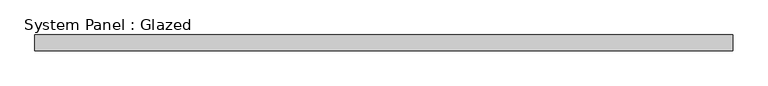
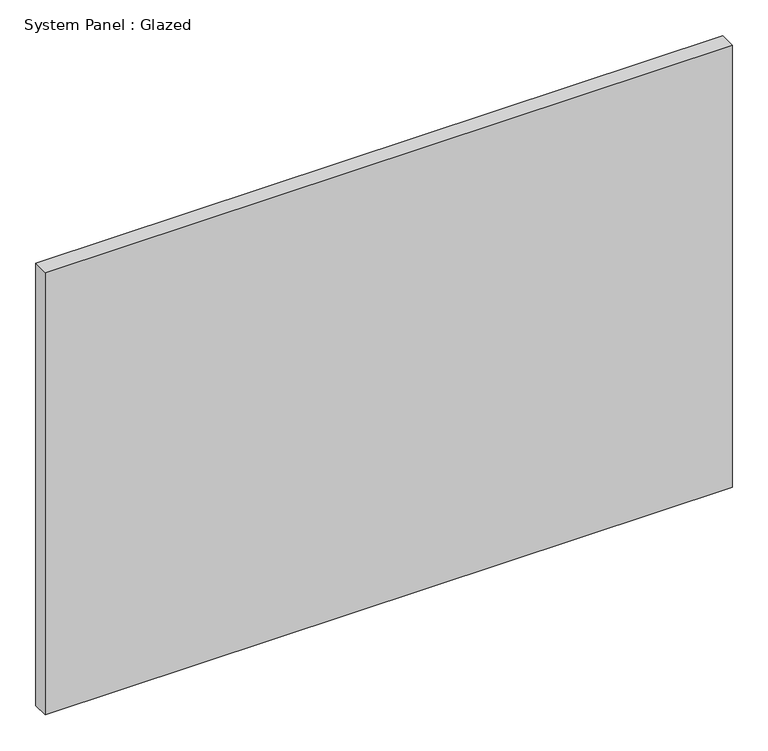
"""IFC4 building model written with IfcOpenShell, lengths in millimetres: plate geometry, System Panel : Glazed."""

from ifc_helpers import new_model, si_unit, origin, origin_with_axes, place, context, project, spatial, polyline, outline, extrude, source, transform, mapped, element, save


def system_panel_glazed_d90ea448(model_context):
    return source(origin(), model_context, "Body", "SweptSolid", [
        extrude(outline(polyline([(551.392122, 19.05), (-551.392122, 19.05), (-551.392122, 44.45), (551.392122, 44.45), (551.392122, 19.05)])), origin_with_axes(), (0.0, 0.0, 1.0), 750.6041168),
    ])


if __name__ == "__main__":
    model = new_model("IFC4")
    model_context = context("Model", 3, world=origin())
    ifc_project = project(units=[si_unit("LENGTHUNIT", "METRE", prefix="MILLI")], contexts=[model_context])
    site = spatial("IfcSite", under=ifc_project)
    building = spatial("IfcBuilding", under=site)
    placement = place(None, origin())
    system_panel_glazed_shape = system_panel_glazed_d90ea448(model_context)
    element("IfcPlate", 1, ObjectType="System Panel : Glazed", at=placement, inside=building, context=model_context, shape_type="MappedRepresentation", body=[
        mapped(system_panel_glazed_shape, transform((0.0, 0.0, 0.0), x_axis=(1.0, 0.0, 0.0), y_axis=(0.0, 1.0, 0.0), z_axis=(0.0, 0.0, 1.0))),
    ])
    save(model, "model.ifc")

# Revit data of these elements
# Type "System Panel : Glazed"
#   Construction Type Id = "GSP4R"
#   Analytic Construction = "1/8 in Pilkington single glazing"
#   Visual Light Transmittance = 0.9
#   Solar Heat Gain Coefficient = 0.86
#   Heat Transfer Coefficient (U) = 1.18115 BTU/(h·ft²·°F)
# Element 1 (IfcPlate, "System Panel : Glazed")
#   Materials on its faces: "Glass"
# Materials
#   "Glass": class "Glass", colour RGB 0 128 192, transparency 0.75, Description = "Soda Lime Glass", Cost = 0
